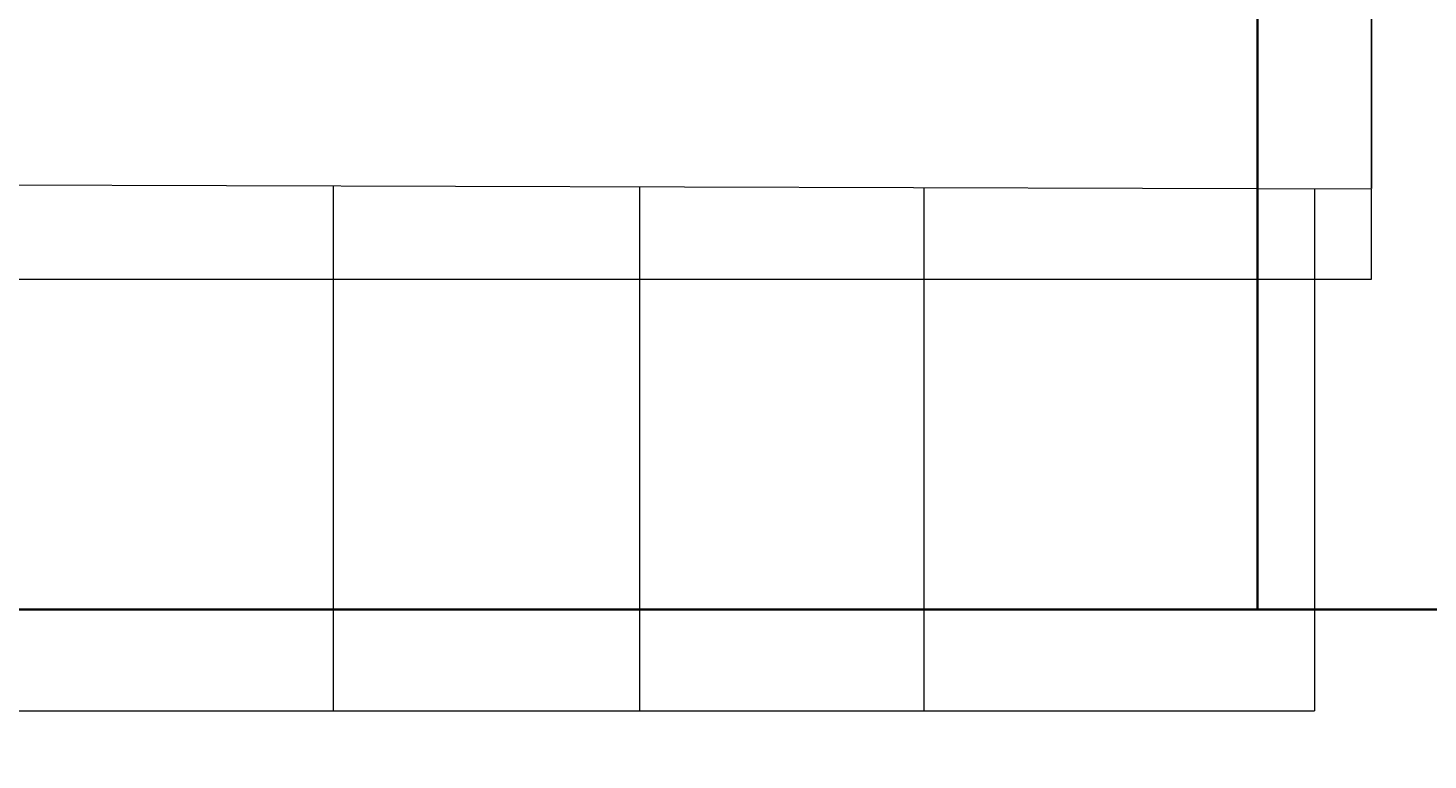
# Model space of a CAD drawing. Units: inches. Extents: x 69 to 650, y -16 to 573.
# Tile 23 of 26: x 383 to 516, y 398 to 467. Entities that reach past the tile are written whole.
import ezdxf

# ---------------------------------------------------------------- set-up
doc = ezdxf.new("R2010")
doc.units = ezdxf.units.IN
doc.header["$MEASUREMENT"] = 0
for name, color, linetype, lineweight in [('A-ANNO-DIMS', 2, 'Continuous', 18), ('A-ELEV', 8, 'Continuous', 18), ('A-WALL', 7, 'Continuous', 35)]:
    doc.layers.add(name, color=color, linetype=linetype, lineweight=lineweight)
doc.styles.get("Standard").update_dxf_attribs({"font": 'arial.ttf'})
doc.dimstyles.get("Standard").update_dxf_attribs({"dimtxt": 0.8125, "dimasz": 0.18, "dimexe": 0.18, "dimexo": 0.0625, "dimgap": 0.09, "dimtad": 0, "dimtih": 1, "dimtoh": 1, "dimdec": 4, "dimzin": 0, "dimdsep": 46, "dimlunit": 4, "dimtxsty": 'Standard', "dimcen": 0.09, "dimadec": 0, "dimazin": 0, "dimtfac": 1, "dimtdec": 4, "dimtofl": 0, "dimtmove": 0, "dimatfit": 3, "dimfxl": 1, "dimtolj": 1, "dimtzin": 0, "dimarcsym": 0})

# ---------------------------------------------------------------- blocks, each defined once
blk = doc.blocks.new('*D19')
at = {"layer": 'A-ANNO-DIMS', "color": 0, "lineweight": -2, "transparency": 16777216}
for p, q in [((99.56, 471.72), (99.56, 572.74)), ((619.56, 87.99), (619.56, 572.74)), ((99.74, 572.56), (358.57, 572.56)), ((619.38, 572.56), (360.54, 572.56))]:
    blk.add_line(p, q, dxfattribs=at)
at = {"layer": 'A-ANNO-DIMS', "color": 0, "transparency": 16777216}
for points in [[(99.74, 572.59), (99.74, 572.53), (99.56, 572.56)], [(619.38, 572.59), (619.38, 572.53), (619.56, 572.56)]]:
    blk.add_solid(points, dxfattribs=at)
at = {"layer": 'Defpoints', "color": 0, "transparency": 16777216}
for p in [(619.56, 572.56), (99.56, 471.66), (619.56, 87.93)]:
    blk.add_point(p, dxfattribs=at)
at = {"layer": 'A-ANNO-DIMS', "color": 0, "transparency": 16777216, "insert": (359.56, 572.56), "char_height": 0.812, "attachment_point": 5}
blk.add_mtext('\\A1;520', dxfattribs=at)
blk = doc.blocks.new('*D20')
at = {"layer": 'A-ANNO-DIMS', "color": 0, "lineweight": -2, "transparency": 16777216}
for p, q in [((504.24, 544.16), (648.14, 544.16)), ((647.96, 543.98), (647.96, 304.55)), ((647.96, 64.11), (647.96, 303.54)), ((619.62, 63.93), (648.14, 63.93))]:
    blk.add_line(p, q, dxfattribs=at)
at = {"layer": 'A-ANNO-DIMS', "color": 0, "transparency": 16777216}
for points in [[(647.93, 543.98), (647.99, 543.98), (647.96, 544.16)], [(647.93, 64.11), (647.99, 64.11), (647.96, 63.93)]]:
    blk.add_solid(points, dxfattribs=at)
at = {"layer": 'Defpoints', "color": 0, "transparency": 16777216}
for p in [(504.18, 544.16), (647.96, 544.16), (619.56, 63.93)]:
    blk.add_point(p, dxfattribs=at)
at = {"layer": 'A-ANNO-DIMS', "color": 0, "transparency": 16777216, "insert": (647.96, 304.04), "char_height": 0.812, "attachment_point": 5}
blk.add_mtext('\\A1;480.2', dxfattribs=at)
blk = doc.blocks.new('*D57')
at = {"layer": 'A-ANNO-DIMS', "color": 0, "lineweight": -2, "transparency": 16777216}
for p, q in [((551.53, 414.41), (648.14, 414.41)), ((647.96, 414.23), (647.96, 413.68)), ((500.33, 411.93), (648.14, 411.93)), ((647.96, 412.11), (647.96, 412.67))]:
    blk.add_line(p, q, dxfattribs=at)
at = {"layer": 'A-ANNO-DIMS', "color": 0, "transparency": 16777216}
for points in [[(647.93, 414.23), (647.99, 414.23), (647.96, 414.41)], [(647.93, 412.11), (647.99, 412.11), (647.96, 411.93)]]:
    blk.add_solid(points, dxfattribs=at)
at = {"layer": 'Defpoints', "color": 0, "transparency": 16777216}
for p in [(551.46, 414.41), (500.26, 411.93), (647.96, 411.93)]:
    blk.add_point(p, dxfattribs=at)
at = {"layer": 'A-ANNO-DIMS', "color": 0, "transparency": 16777216, "insert": (647.96, 413.17), "char_height": 0.812, "attachment_point": 5}
blk.add_mtext('\\A1;2.48', dxfattribs=at)
blk = doc.blocks.new('*D62')
at = {"layer": 'A-ANNO-DIMS', "color": 0, "lineweight": -2, "transparency": 16777216}
for p, q in [((204.87, 452.8), (204.87, 572.74)), ((511.09, 451.98), (511.09, 572.74)), ((205.05, 572.56), (356.52, 572.56)), ((510.91, 572.56), (359.44, 572.56))]:
    blk.add_line(p, q, dxfattribs=at)
at = {"layer": 'A-ANNO-DIMS', "color": 0, "transparency": 16777216}
for points in [[(205.05, 572.59), (205.05, 572.53), (204.87, 572.56)], [(510.91, 572.59), (510.91, 572.53), (511.09, 572.56)]]:
    blk.add_solid(points, dxfattribs=at)
at = {"layer": 'Defpoints', "color": 0, "transparency": 16777216}
for p in [(511.09, 572.56), (204.87, 452.74), (511.09, 451.92)]:
    blk.add_point(p, dxfattribs=at)
at = {"layer": 'A-ANNO-DIMS', "color": 0, "transparency": 16777216, "insert": (357.98, 572.56), "char_height": 0.812, "attachment_point": 5}
blk.add_mtext('\\A1;306.2', dxfattribs=at)

msp = doc.modelspace()

# ---------------------------------------------------------------- linework, layer by layer
at = {"layer": 'A-ELEV'}
for p, q in [((511.0913, 451.9213), (218.848, 452.7384)), ((412.3358, 452.1974), (412.3358, 402.3042)), ((441.4701, 452.116), (441.4701, 402.3042)), ((468.5246, 452.0403), (468.5246, 402.3042)), ((505.6709, 451.9365), (505.6709, 402.3042)), ((511.0913, 443.3425), (511.0913, 451.9213)), ((204.8658, 443.3425), (511.0913, 443.3425)), ((214.8863, 402.3042), (505.6709, 402.3042))]:
    msp.add_line(p, q, dxfattribs=at)
at = {"layer": 'A-WALL'}
for p, q in [((500.263, 411.93), (500.263, 533.4142)), ((99.556, 411.93), (619.555, 411.93))]:
    msp.add_line(p, q, dxfattribs=at)

# ---------------------------------------------------------------- dimensions: what is measured, and where the dimension line sits
at = {"layer": 'A-ANNO-DIMS'}
for base, p1, p2, override, picture, middle in [((619.555, 572.5573), (99.556, 471.6595), (619.555, 87.93), {"dimdec": 0, "dimlfac": 1, "dimrnd": 0, "dimzin": 0, "dimdsep": 46, "dimlunit": 2}, '*D19', (359.5555, 572.5573)), ((511.0913, 572.5573), (204.8658, 452.7384), (511.0913, 451.9213), {"dimdec": 1, "dimlfac": 1, "dimrnd": 0, "dimzin": 0, "dimdsep": 46, "dimlunit": 2}, '*D62', (357.9786, 572.5573))]:
    dim = msp.add_linear_dim(base=base, p1=p1, p2=p2, dimstyle='Standard', override=override, dxfattribs=at)
    dim.commit()
    dim.dimension.update_dxf_attribs({"geometry": picture, "text_midpoint": middle})
for base, p1, p2, override, picture, middle in [((647.955, 544.1573), (619.555, 63.93), (504.1763, 544.1573), {"dimdec": 1, "dimlfac": 1, "dimrnd": 0, "dimzin": 0, "dimdsep": 46, "dimlunit": 2}, '*D20', (647.955, 304.0436)), ((647.955, 411.93), (551.4641, 414.4146), (500.263, 411.93), {"dimdec": 2, "dimlfac": 1, "dimrnd": 0, "dimzin": 0, "dimdsep": 46, "dimlunit": 2}, '*D57', (647.955, 413.1723))]:
    dim = msp.add_linear_dim(base=base, p1=p1, p2=p2, angle=90, dimstyle='Standard', override=override, dxfattribs=at)
    dim.commit()
    dim.dimension.update_dxf_attribs({"geometry": picture, "text_midpoint": middle})

doc.saveas('drawing.dxf')
